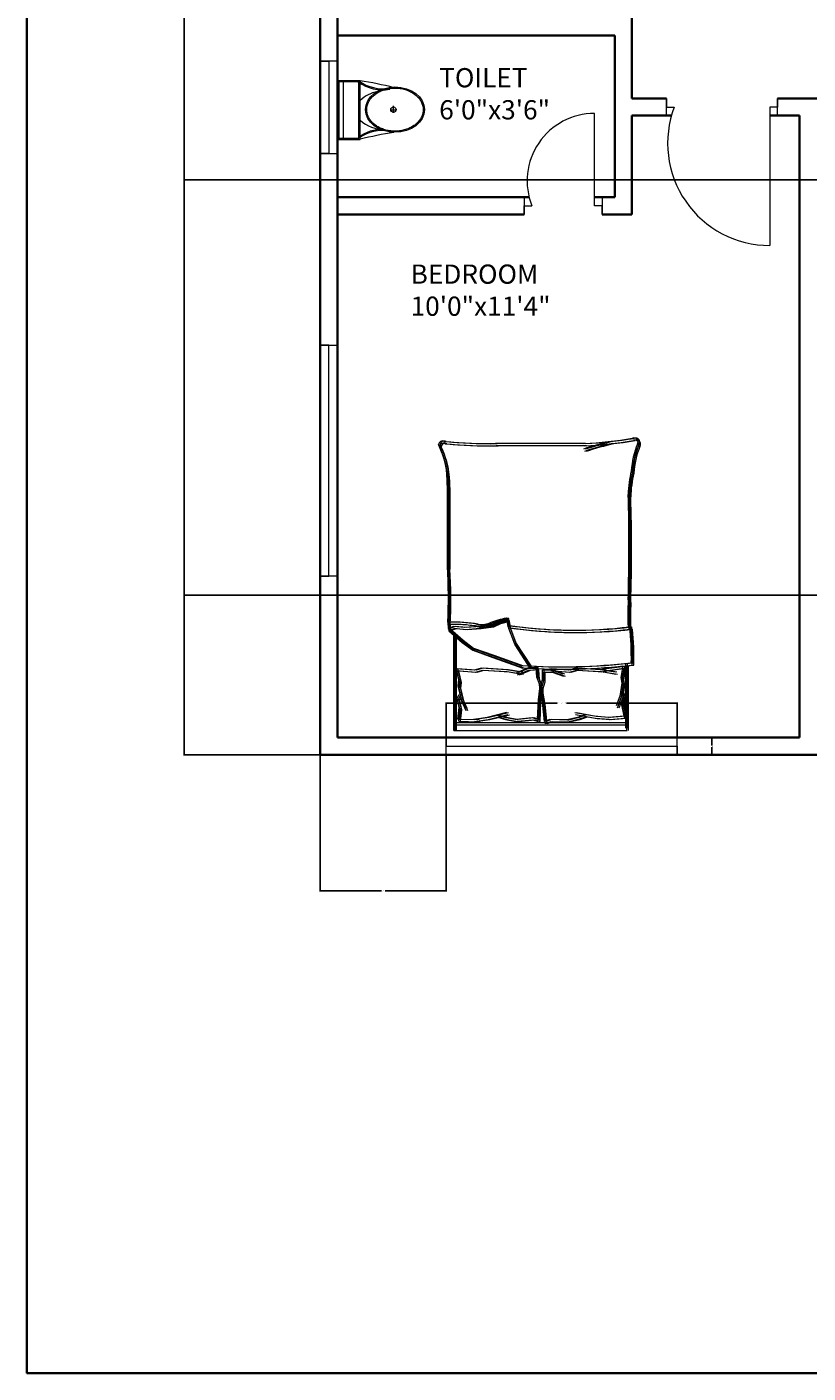
# Model space of a CAD drawing. Units: inches. Extents: x 2234 to 3001, y 1541 to 2386.
# Tile 1 of 12: x 2234 to 2437, y 1541 to 1891. Entities that reach past the tile are written whole.
import ezdxf

# ---------------------------------------------------------------- set-up
doc = ezdxf.new("R2010")
doc.units = ezdxf.units.IN
for name, color, linetype, lineweight in [('A-ANNO-DIMS', 2, 'Continuous', 18), ('A-ANNO-TTLB', 7, 'Continuous', 35), ('A-AREA-IDEN', 7, 'Continuous', 18), ('A-DOOR', 3, 'Continuous', 18), ('A-FLOR-FIXT', 9, 'Continuous', 18), ('A-FURN', 9, 'Continuous', 13), ('A-GLAZ', 4, 'Continuous', 18), ('A-WALL', 7, 'Continuous', 35)]:
    doc.layers.add(name, color=color, linetype=linetype, lineweight=lineweight)
doc.styles.get("Standard").update_dxf_attribs({"font": 'arial.ttf'})
doc.dimstyles.get("Standard").update_dxf_attribs({"dimtxt": 0.18, "dimasz": 0.18, "dimexe": 0.18, "dimexo": 0.0625, "dimgap": 0.09, "dimtad": 0, "dimtih": 1, "dimtoh": 1, "dimdec": 4, "dimzin": 0, "dimdsep": 46, "dimtxsty": 'Standard', "dimcen": 0.09, "dimadec": 0, "dimazin": 0, "dimtfac": 1, "dimtdec": 4, "dimtofl": 0, "dimtmove": 0, "dimatfit": 3, "dimfxl": 1, "dimtolj": 1, "dimtzin": 0, "dimarcsym": 0})

# ---------------------------------------------------------------- blocks, each defined once
blk = doc.blocks.new('A$C31115884')
for p, q in [((283, 498), (223, 498)), ((258, 466), (258, 523)), ((0, 200), (0, 0)), ((520, 200), (0, 200)), ((10, 190), (10, 10)), ((510, 190), (10, 190)), ((510, 10), (510, 190)), ((520, 0), (520, 200)), ((510, 54), (0, 54)), ((10, 10), (510, 10)), ((0, 0), (520, 0))]:
    blk.add_line(p, q)
blk.add_circle((256, 496), 23.6)
for centre, radius, start, end in [((2778, -205), 2807, 165.4549, 171.7133), ((3237, 905), 2807, 188.2867, 194.5451), ((-295, 403), 365, 324.2091, 9.3499), ((-295, 403), 375, 324.2091, 9.3499), ((139, 406), 293, 315.8436, 2.6563), ((806, 403), 375, 179.2036, 215.7909), ((806, 403), 365, 170.6501, 215.7909), ((384, 406), 293, 190.2774, 224.1564)]:
    blk.add_arc(centre, radius, start, end)
blk.add_ellipse((256, 510), major_axis=(0, -261), ratio=0.772727)
blk.add_open_spline([(256, 259), (263, 259), (270, 260), (288, 262), (299, 265), (320, 273), (330, 278), (350, 291), (360, 299), (378, 316), (386, 326), (402, 347), (409, 358), (421, 383), (427, 395), (436, 422), (440, 436), (445, 465), (447, 480), (448, 509), (448, 524), (445, 553), (443, 568), (436, 596), (432, 610), (422, 636), (416, 649), (402, 672), (395, 683), (379, 703), (370, 712), (351, 728), (341, 735), (321, 746), (310, 751), (289, 757), (278, 759), (256, 761), (245, 761), (223, 757), (212, 754), (191, 746), (181, 741), (161, 728), (151, 720), (133, 703), (125, 693), (110, 672), (103, 660), (90, 636), (85, 623), (76, 596), (72, 582), (67, 553), (66, 538), (64, 509), (65, 494), (68, 465), (70, 450), (77, 422), (81, 408), (91, 382), (97, 370), (111, 346), (118, 335), (135, 316), (144, 307), (162, 291), (172, 284), (193, 273), (203, 269), (225, 262), (236, 260), (250, 259), (253, 259), (256, 259)], degree=3, knots=[0, 0, 0, 0, 0.110105, 0.110105, 0.285049, 0.285049, 0.459994, 0.459994, 0.634938, 0.634938, 0.809882, 0.809882, 0.984827, 0.984827, 1.159771, 1.159771, 1.334715, 1.334715, 1.50966, 1.50966, 1.684604, 1.684604, 1.859549, 1.859549, 2.034493, 2.034493, 2.209437, 2.209437, 2.384382, 2.384382, 2.559326, 2.559326, 2.73427, 2.73427, 2.909215, 2.909215, 3.084159, 3.084159, 3.259103, 3.259103, 3.434048, 3.434048, 3.608992, 3.608992, 3.783936, 3.783936, 3.958881, 3.958881, 4.133825, 4.133825, 4.30877, 4.30877, 4.483714, 4.483714, 4.658658, 4.658658, 4.833603, 4.833603, 5.008547, 5.008547, 5.183491, 5.183491, 5.358436, 5.358436, 5.53338, 5.53338, 5.708324, 5.708324, 5.883269, 5.883269, 6.058213, 6.058213, 6.233158, 6.233158, 6.283185, 6.283185, 6.283185, 6.283185])
blk = doc.blocks.new('WIN-60-A')
for p, q in [((0, 60), (4.5, 60)), ((4.5, 60), (2.25, 60)), ((2.25, 60), (2.25, 0)), ((2.25, 0), (0, 0)), ((0, 0), (4.5, 0))]:
    blk.add_line(p, q)
blk = doc.blocks.new('WIN-60-B')
for p, q in [((0, 60), (4.5, 60)), ((4.5, 60), (2.25, 60)), ((2.25, 60), (2.25, 0)), ((4.5, 0), (0, 0)), ((2.25, 0), (4.5, 0))]:
    blk.add_line(p, q)
blk = doc.blocks.new('WIN-24-B')
for p, q in [((4.5, 24), (0, 24)), ((0, 24), (2.25, 24)), ((2.25, 24), (2.25, 0)), ((2.25, 0), (0, 0)), ((0, 0), (4.5, 0))]:
    blk.add_line(p, q)
blk = doc.blocks.new('BED-DOUBLE-B')
for p, q in [((37.77, 74.61), (14.78, 74.61)), ((37.77, 74.61), (14.78, 74.61)), ((37.98, 74.02), (15, 74.02)), ((37.98, 74.02), (15, 74.02)), ((38.22, 74.59), (15.24, 74.59)), ((38.22, 74.59), (15.24, 74.59)), ((38.44, 73.99), (15.45, 73.99)), ((38.44, 73.99), (15.46, 73.99)), ((2.39, 28.15), (2.47, 26.53, 3.61)), ((2.39, 28.15), (2.47, 26.53, 3.61)), ((2.85, 28.13), (2.92, 26.5, 3.61)), ((2.85, 28.13), (2.93, 26.5, 3.61)), ((15.47, 28.4), (13.59, 27.54)), ((15.47, 28.4), (13.59, 27.54)), ((15.93, 28.38), (14.05, 27.52)), ((15.93, 28.38), (14.05, 27.52)), ((17.79, 28.98), (15.47, 28.4)), ((17.79, 28.98), (15.47, 28.4)), ((18, 28.38), (15.68, 27.81)), ((18, 28.38), (15.69, 27.81)), ((18.24, 28.96), (15.93, 28.38)), ((18.24, 28.96), (15.93, 28.38)), ((18.46, 28.36), (16.14, 27.79)), ((18.46, 28.36), (16.14, 27.79)), ((18.07, 27.1), (17.79, 28.98)), ((18.07, 27.1), (17.79, 28.98)), ((18.29, 26.51), (18, 28.38)), ((18.29, 26.51), (18, 28.38)), ((18.53, 27.08), (18.24, 28.96)), ((18.53, 27.08), (18.24, 28.96)), ((18.75, 26.49), (18.46, 28.36)), ((18.75, 26.49), (18.46, 28.36)), ((3.9, 27.1), (2.47, 26.53)), ((3.9, 27.1), (2.47, 26.53)), ((2.47, 26.53), (5.93, 23.49)), ((2.47, 26.53), (5.93, 23.49)), ((2.61, 27.56), (2.68, 25.93, 3.61)), ((2.61, 27.56), (2.68, 25.93, 3.61)), ((4.12, 26.51), (2.68, 25.93)), ((4.12, 26.51), (2.68, 25.93)), ((2.68, 25.93), (6.14, 22.89)), ((2.68, 25.93), (6.14, 22.89)), ((4.36, 27.08), (2.92, 26.5)), ((2.92, 26.5), (6.38, 23.47)), ((4.36, 27.08), (2.93, 26.5)), ((2.93, 26.5), (6.39, 23.47)), ((3.06, 27.54), (3.14, 25.91, 3.61)), ((3.06, 27.54), (3.14, 25.91, 3.61)), ((4.57, 26.49), (3.14, 25.91)), ((4.57, 26.49), (3.14, 25.91)), ((3.14, 25.91), (6.6, 22.87)), ((3.14, 25.91), (6.6, 22.87)), ((6.79, 26.81), (3.9, 27.1)), ((6.8, 26.81), (3.9, 27.1)), ((3.96, 0.62), (3.96, 25.46)), ((3.96, 0.62), (3.96, 25.46)), ((7.01, 26.22), (4.12, 26.51)), ((7.01, 26.22), (4.12, 26.51)), ((4.18, 0.02), (4.18, 24.87)), ((4.18, 0.02), (4.18, 24.87)), ((7.25, 26.79), (4.36, 27.08)), ((7.25, 26.79), (4.36, 27.08)), ((4.42, 0.6), (4.42, 25.44)), ((4.42, 0.6), (4.42, 25.44)), ((7.47, 26.2), (4.57, 26.49)), ((7.47, 26.2), (4.57, 26.49)), ((4.63, 0), (4.63, 24.85)), ((4.63, 0), (4.63, 24.85)), ((10.41, 27.1), (6.79, 26.81)), ((10.41, 27.1), (6.8, 26.81)), ((10.62, 26.51), (7.01, 26.22)), ((10.62, 26.51), (7.01, 26.22)), ((10.87, 27.08), (7.25, 26.79)), ((10.87, 27.08), (7.25, 26.79)), ((11.08, 26.49), (7.47, 26.2)), ((11.08, 26.49), (7.47, 26.2)), ((13.59, 27.54), (10.41, 27.1)), ((13.59, 27.54), (10.41, 27.1)), ((13.8, 26.94), (10.62, 26.51)), ((13.81, 26.94), (10.62, 26.51)), ((14.05, 27.52), (10.87, 27.08)), ((14.05, 27.52), (10.87, 27.08)), ((14.26, 26.92), (11.08, 26.49)), ((14.26, 26.92), (11.08, 26.49)), ((15.68, 27.81), (13.8, 26.94)), ((15.69, 27.81), (13.81, 26.94)), ((16.14, 27.79), (14.26, 26.92)), ((16.14, 27.79), (14.26, 26.92)), ((19.67, 22.91), (18.07, 27.1)), ((19.67, 22.91), (18.07, 27.1)), ((19.88, 22.32), (18.29, 26.51)), ((19.88, 22.32), (18.29, 26.51)), ((20.12, 22.89), (18.53, 27.08)), ((20.12, 22.89), (18.53, 27.08)), ((20.34, 22.29), (18.75, 26.49)), ((20.34, 22.29), (18.75, 26.49)), ((5.93, 23.49), (8.67, 21.47)), ((5.93, 23.49), (8.68, 21.47)), ((6.14, 22.89), (8.89, 20.87)), ((6.14, 22.89), (8.89, 20.87)), ((6.38, 23.47), (9.13, 21.45)), ((6.39, 23.47), (9.13, 21.45)), ((6.6, 22.87), (9.35, 20.85)), ((6.6, 22.87), (9.35, 20.85)), ((8.67, 21.47), (13.88, 19.59)), ((8.68, 21.47), (13.88, 19.59)), ((9.13, 21.45), (14.34, 19.57)), ((9.13, 21.45), (14.34, 19.57)), ((23.58, 16.85), (19.67, 22.91)), ((23.58, 16.85), (19.67, 22.91)), ((23.79, 16.25), (19.88, 22.32)), ((23.79, 16.25), (19.88, 22.32)), ((24.04, 16.83), (20.12, 22.89)), ((24.04, 16.83), (20.12, 22.89)), ((24.25, 16.23), (20.34, 22.29)), ((24.25, 16.23), (20.34, 22.29)), ((8.89, 20.87), (14.09, 18.99)), ((8.89, 20.87), (14.09, 18.99)), ((9.35, 20.85), (14.55, 18.97)), ((9.35, 20.85), (14.55, 18.97)), ((13.88, 19.59), (21.67, 16.85)), ((13.88, 19.59), (21.67, 16.85)), ((14.09, 18.99), (21.88, 16.25)), ((14.09, 18.99), (21.88, 16.25)), ((14.34, 19.57), (22.12, 16.83)), ((14.34, 19.57), (22.12, 16.83)), ((14.55, 18.97), (22.34, 16.23)), ((14.55, 18.97), (22.34, 16.23)), ((48.59, 17.53), (48.59, 0.62)), ((48.59, 17.53), (48.59, 0.62)), ((49.05, 17.51), (49.05, 0.6)), ((49.05, 17.51), (49.05, 0.6)), ((9.28, 15.72), (4.49, 16.09)), ((4.49, 16.09), (5.22, 13.16)), ((9.29, 15.72), (4.49, 16.09)), ((4.49, 16.09), (5.22, 13.16)), ((9.5, 15.12), (4.71, 15.5)), ((4.71, 15.5), (5.43, 12.56)), ((9.5, 15.12), (4.71, 15.5)), ((4.71, 15.5), (5.43, 12.56)), ((9.74, 15.69), (4.95, 16.07)), ((4.95, 16.07), (5.67, 13.14)), ((9.74, 15.69), (4.95, 16.07)), ((4.95, 16.07), (5.67, 13.14)), ((9.96, 15.1), (5.16, 15.47)), ((5.16, 15.47), (5.89, 12.54)), ((9.96, 15.1), (5.16, 15.47)), ((5.16, 15.47), (5.89, 12.54)), ((11.12, 16.24), (9.28, 15.72)), ((11.12, 16.24), (9.29, 15.72)), ((11.33, 15.64), (9.5, 15.12)), ((11.33, 15.64), (9.5, 15.12)), ((11.57, 16.21), (9.74, 15.69)), ((11.57, 16.21), (9.74, 15.69)), ((11.79, 15.62), (9.96, 15.1)), ((11.79, 15.62), (9.96, 15.1)), ((17.66, 15.83), (11.12, 16.24)), ((17.66, 15.83), (11.12, 16.24)), ((17.87, 15.24), (11.33, 15.64)), ((17.87, 15.24), (11.33, 15.64)), ((18.12, 15.81), (11.57, 16.21)), ((18.12, 15.81), (11.57, 16.21)), ((18.33, 15.22), (11.79, 15.62)), ((18.33, 15.22), (11.79, 15.62)), ((21.43, 15.21), (17.66, 15.83)), ((21.43, 15.21), (17.66, 15.83)), ((21.64, 14.61), (17.87, 15.24)), ((21.64, 14.61), (17.87, 15.24)), ((21.88, 15.19), (18.12, 15.81)), ((21.88, 15.19), (18.12, 15.81)), ((22.1, 14.59), (18.33, 15.22)), ((22.1, 14.59), (18.33, 15.22)), ((23.12, 16.25), (20.25, 15.05)), ((23.12, 16.25), (20.25, 15.05)), ((23.33, 15.65), (20.47, 14.45)), ((23.33, 15.65), (20.47, 14.45)), ((23.58, 16.23), (20.71, 15.03)), ((23.58, 16.23), (20.71, 15.03)), ((23.79, 15.63), (20.92, 14.43)), ((23.79, 15.63), (20.92, 14.43)), ((25.41, 16.39), (23.12, 16.25)), ((25.41, 16.39), (23.12, 16.25)), ((25.62, 15.79), (23.33, 15.65)), ((25.62, 15.79), (23.33, 15.65)), ((25.87, 16.37), (23.58, 16.23)), ((25.87, 16.37), (23.58, 16.23)), ((26.08, 15.77), (23.79, 15.63)), ((26.08, 15.77), (23.79, 15.63)), ((25.57, 13.89), (25.41, 16.39)), ((25.57, 13.89), (25.41, 16.39)), ((25.78, 13.3), (25.62, 15.79)), ((25.78, 13.3), (25.62, 15.79)), ((26.02, 13.87), (25.87, 16.37)), ((26.02, 13.87), (25.87, 16.37)), ((26.24, 13.27), (26.08, 15.77)), ((26.24, 13.27), (26.08, 15.77)), ((27.03, 13.3), (27.03, 15.8)), ((27.03, 15.8), (29.33, 15.8)), ((27.03, 13.3), (27.03, 15.8)), ((27.03, 15.8), (29.33, 15.8)), ((27.24, 12.7), (27.24, 15.21)), ((27.24, 15.21), (29.54, 15.21)), ((27.24, 12.7), (27.24, 15.21)), ((27.24, 15.21), (29.54, 15.21)), ((27.49, 13.28), (27.49, 15.78)), ((27.49, 15.78), (29.78, 15.78)), ((27.49, 13.28), (27.49, 15.78)), ((27.49, 15.78), (29.78, 15.78)), ((27.7, 12.68), (27.7, 15.19)), ((27.7, 15.19), (30, 15.19)), ((27.7, 12.68), (27.7, 15.19)), ((27.7, 15.19), (30, 15.19)), ((33.73, 15.72), (28.94, 16.09)), ((33.73, 15.72), (28.94, 16.09)), ((33.95, 15.12), (29.15, 15.5)), ((33.95, 15.12), (29.15, 15.5)), ((29.33, 15.8), (32.26, 14.78)), ((29.33, 15.8), (32.26, 14.78)), ((34.19, 15.69), (29.4, 16.07)), ((34.19, 15.69), (29.4, 16.07)), ((29.54, 15.21), (32.48, 14.19)), ((29.54, 15.21), (32.48, 14.19)), ((34.4, 15.1), (29.61, 15.47)), ((34.4, 15.1), (29.61, 15.47)), ((29.78, 15.78), (32.72, 14.76)), ((29.78, 15.78), (32.72, 14.76)), ((30, 15.19), (32.93, 14.17)), ((30, 15.19), (32.93, 14.17)), ((35.56, 16.24), (33.73, 15.72)), ((35.56, 16.24), (33.73, 15.72)), ((35.78, 15.64), (33.95, 15.12)), ((35.78, 15.64), (33.95, 15.12)), ((36.02, 16.21), (34.19, 15.69)), ((36.02, 16.21), (34.19, 15.69)), ((36.23, 15.62), (34.4, 15.1)), ((36.23, 15.62), (34.4, 15.1)), ((42.11, 15.83), (35.56, 16.24)), ((42.11, 15.83), (35.56, 16.24)), ((42.32, 15.24), (35.78, 15.64)), ((42.32, 15.24), (35.78, 15.64)), ((42.57, 15.81), (36.02, 16.21)), ((42.57, 15.81), (36.02, 16.21)), ((42.78, 15.22), (36.23, 15.62)), ((42.78, 15.22), (36.23, 15.62)), ((42.11, 15.83), (43.17, 16.13)), ((42.11, 15.83), (43.17, 16.13)), ((45.87, 15.21), (42.11, 15.83)), ((45.87, 15.21), (42.11, 15.83)), ((42.32, 15.24), (43.38, 15.54)), ((42.32, 15.24), (43.38, 15.54)), ((46.09, 14.61), (42.32, 15.24)), ((46.09, 14.61), (42.32, 15.24)), ((42.57, 15.81), (43.62, 16.11)), ((42.57, 15.81), (43.62, 16.11)), ((46.33, 15.19), (42.57, 15.81)), ((46.33, 15.19), (42.57, 15.81)), ((42.78, 15.22), (43.84, 15.52)), ((42.78, 15.22), (43.84, 15.52)), ((46.54, 14.59), (42.78, 15.22)), ((46.54, 14.59), (42.78, 15.22)), ((43.17, 16.13), (47.93, 16.81)), ((43.17, 16.13), (47.93, 16.81)), ((43.38, 15.54), (48.14, 16.21)), ((43.38, 15.54), (48.14, 16.21)), ((43.62, 16.11), (48.38, 16.79)), ((43.62, 16.11), (48.38, 16.79)), ((43.84, 15.52), (48.6, 16.19)), ((43.84, 15.52), (48.6, 16.19)), ((47.93, 16.81), (47.39, 13.84)), ((47.93, 16.81), (47.39, 13.84)), ((48.14, 16.21), (47.6, 13.24)), ((48.14, 16.21), (47.6, 13.24)), ((48.38, 16.79), (47.84, 13.82)), ((48.38, 16.79), (47.84, 13.82)), ((48.6, 16.19), (48.06, 13.22)), ((48.6, 16.19), (48.06, 13.22)), ((48.8, 16.93), (48.8, 0.02)), ((48.8, 16.93), (48.8, 0.02)), ((49.26, 16.91), (49.26, 0)), ((49.26, 16.91), (49.26, 0)), ((5.22, 13.16), (5.04, 11.66)), ((5.22, 13.16), (5.04, 11.66)), ((5.04, 11.66), (5.79, 8.33)), ((5.04, 11.66), (5.79, 8.33)), ((5.43, 12.56), (5.25, 11.07)), ((5.43, 12.56), (5.25, 11.07)), ((5.25, 11.07), (6, 7.73)), ((5.25, 11.07), (6, 7.73)), ((5.67, 13.14), (5.5, 11.64)), ((5.67, 13.14), (5.5, 11.64)), ((5.5, 11.64), (6.25, 8.31)), ((5.5, 11.64), (6.25, 8.31)), ((5.89, 12.54), (5.71, 11.04)), ((5.89, 12.54), (5.71, 11.04)), ((5.71, 11.04), (6.46, 7.71)), ((5.71, 11.04), (6.46, 7.71)), ((26.21, 12.17), (25.57, 13.89)), ((26.21, 12.17), (25.57, 13.89)), ((26.43, 11.58), (25.78, 13.3)), ((26.43, 11.58), (25.78, 13.3)), ((25.94, 7.96), (26.29, 10.96)), ((25.94, 7.96), (26.29, 10.96)), ((26.67, 12.15), (26.02, 13.87)), ((26.67, 12.15), (26.02, 13.87)), ((26.29, 10.96), (26.21, 12.17)), ((26.29, 10.96), (26.21, 12.17)), ((26.88, 11.56), (26.24, 13.27)), ((26.89, 11.56), (26.24, 13.27)), ((26.39, 7.94), (26.75, 10.94)), ((26.39, 7.94), (26.75, 10.94)), ((26.5, 10.36), (26.43, 11.58)), ((26.5, 10.36), (26.43, 11.58)), ((26.49, 11.54), (27.03, 13.3)), ((26.49, 11.54), (27.03, 13.3)), ((26.49, 10.33), (26.49, 11.54)), ((26.49, 10.33), (26.49, 11.54)), ((26.75, 10.94), (26.67, 12.15)), ((26.75, 10.94), (26.67, 12.15)), ((26.7, 10.95), (27.24, 12.7)), ((26.7, 10.95), (27.24, 12.7)), ((26.7, 9.73), (26.7, 10.95)), ((26.7, 9.73), (26.7, 10.95)), ((26.96, 10.34), (26.88, 11.56)), ((26.96, 10.34), (26.89, 11.56)), ((26.95, 11.52), (27.49, 13.28)), ((26.95, 11.52), (27.49, 13.28)), ((26.95, 10.31), (26.95, 11.52)), ((26.95, 10.31), (26.95, 11.52)), ((27.16, 10.93), (27.7, 12.68)), ((27.16, 10.93), (27.7, 12.68)), ((27.16, 9.71), (27.16, 10.93)), ((27.16, 9.71), (27.16, 10.93)), ((47.66, 12.35), (47.12, 8.98)), ((47.66, 12.35), (47.12, 8.98)), ((47.87, 11.76), (47.33, 8.38)), ((47.87, 11.76), (47.33, 8.38)), ((47.39, 13.84), (47.66, 12.35)), ((47.39, 13.84), (47.66, 12.35)), ((48.11, 12.33), (47.57, 8.96)), ((48.11, 12.33), (47.57, 8.96)), ((47.6, 13.24), (47.87, 11.76)), ((47.6, 13.24), (47.87, 11.76)), ((48.33, 11.74), (47.79, 8.36)), ((48.33, 11.74), (47.79, 8.36)), ((47.84, 13.82), (48.11, 12.33)), ((47.84, 13.82), (48.11, 12.33)), ((48.06, 13.22), (48.33, 11.74)), ((48.06, 13.22), (48.33, 11.74)), ((4.84, 8.4), (5.32, 9.38)), ((4.84, 8.4), (5.32, 9.38)), ((5.39, 6), (4.84, 8.4)), ((5.39, 6), (4.84, 8.4)), ((5.05, 7.81), (5.53, 8.78)), ((5.05, 7.81), (5.53, 8.78)), ((5.61, 5.41), (5.05, 7.81)), ((5.61, 5.41), (5.05, 7.81)), ((5.3, 8.38), (5.78, 9.36)), ((5.3, 8.38), (5.78, 9.36)), ((5.85, 5.98), (5.3, 8.38)), ((5.85, 5.98), (5.3, 8.38)), ((5.51, 7.79), (5.99, 8.76)), ((5.51, 7.79), (5.99, 8.76)), ((6.06, 5.39), (5.51, 7.79)), ((6.07, 5.39), (5.51, 7.79)), ((5.79, 8.33), (6.89, 5.83)), ((5.79, 8.33), (6.89, 5.83)), ((6, 7.73), (7.11, 5.23)), ((6, 7.73), (7.11, 5.23)), ((6.25, 8.31), (7.35, 5.81)), ((6.25, 8.31), (7.35, 5.81)), ((6.46, 7.71), (7.56, 5.21)), ((6.46, 7.71), (7.56, 5.21)), ((25.71, 2.94), (25.94, 7.96)), ((25.71, 2.94), (25.94, 7.96)), ((25.92, 2.35), (26.15, 7.37)), ((25.92, 2.35), (26.15, 7.37)), ((26.15, 7.37), (26.5, 10.36)), ((26.15, 7.37), (26.5, 10.36)), ((26.17, 2.92), (26.39, 7.94)), ((26.17, 2.92), (26.39, 7.94)), ((26.38, 2.33), (26.61, 7.35)), ((26.38, 2.33), (26.61, 7.35)), ((27.03, 7.36), (26.49, 10.33)), ((27.03, 7.36), (26.49, 10.33)), ((26.61, 7.35), (26.96, 10.34)), ((26.61, 7.35), (26.96, 10.34)), ((27.24, 6.76), (26.7, 9.73)), ((27.24, 6.76), (26.7, 9.73)), ((27.49, 7.34), (26.95, 10.31)), ((27.49, 7.34), (26.95, 10.31)), ((27.57, 2.36), (27.03, 7.36)), ((27.57, 2.36), (27.03, 7.36)), ((27.7, 6.74), (27.16, 9.71)), ((27.7, 6.74), (27.16, 9.71)), ((28.03, 2.34), (27.49, 7.34)), ((28.03, 2.34), (27.49, 7.34)), ((47.12, 8.98), (46.17, 6.41)), ((47.12, 8.98), (46.17, 6.41)), ((47.33, 8.38), (46.38, 5.82)), ((47.33, 8.38), (46.38, 5.82)), ((47.57, 8.96), (46.63, 6.39)), ((47.57, 8.96), (46.63, 6.39)), ((47.79, 8.36), (46.84, 5.8)), ((47.79, 8.36), (46.84, 5.8)), ((48.06, 9.11), (47.52, 10.06)), ((48.06, 9.11), (47.52, 10.06)), ((47.66, 6.68), (48.06, 9.11)), ((47.66, 6.68), (48.06, 9.11)), ((48.27, 8.52), (47.73, 9.46)), ((48.27, 8.52), (47.73, 9.46)), ((47.87, 6.09), (48.27, 8.52)), ((47.87, 6.09), (48.27, 8.52)), ((48.52, 9.09), (47.98, 10.04)), ((48.52, 9.09), (47.98, 10.04)), ((48.11, 6.66), (48.52, 9.09)), ((48.11, 6.66), (48.52, 9.09)), ((48.73, 8.5), (48.19, 9.44)), ((48.73, 8.5), (48.19, 9.44)), ((48.33, 6.07), (48.73, 8.5)), ((48.33, 6.07), (48.73, 8.5)), ((5.04, 3.01), (5.39, 6)), ((5.04, 3.01), (5.39, 6)), ((5.25, 2.41), (5.61, 5.41)), ((5.25, 2.41), (5.61, 5.41)), ((5.5, 2.98), (5.85, 5.98)), ((5.5, 2.98), (5.85, 5.98)), ((5.71, 2.39), (6.06, 5.39)), ((5.71, 2.39), (6.07, 5.39)), ((12.69, 3.48), (17.76, 4.75)), ((12.7, 3.48), (17.76, 4.75)), ((12.91, 2.89), (17.97, 4.15)), ((12.91, 2.89), (17.97, 4.15)), ((13.15, 3.46), (18.21, 4.73)), ((13.15, 3.46), (18.21, 4.73)), ((13.37, 2.87), (18.43, 4.13)), ((13.37, 2.87), (18.43, 4.13)), ((15.23, 4.05), (17.16, 3.49)), ((15.23, 4.05), (17.16, 3.49)), ((15.69, 4.03), (17.61, 3.47)), ((15.69, 4.03), (17.62, 3.47)), ((27.78, 1.77), (27.24, 6.76)), ((27.78, 1.77), (27.24, 6.76)), ((28.24, 1.75), (27.7, 6.74)), ((28.24, 1.75), (27.7, 6.74)), ((40.53, 3.71), (35.4, 4.66)), ((40.53, 3.71), (35.4, 4.66)), ((40.74, 3.12), (35.61, 4.06)), ((40.74, 3.12), (35.61, 4.06)), ((40.98, 3.69), (35.85, 4.64)), ((40.98, 3.69), (35.85, 4.64)), ((37.96, 4.12), (36.07, 3.44)), ((37.96, 4.12), (36.07, 3.44)), ((41.2, 3.1), (36.07, 4.04)), ((41.2, 3.1), (36.07, 4.04)), ((38.17, 3.52), (36.29, 2.85)), ((38.18, 3.52), (36.29, 2.85)), ((38.42, 4.1), (36.53, 3.42)), ((38.42, 4.1), (36.53, 3.42)), ((38.63, 3.5), (36.74, 2.83)), ((38.63, 3.5), (36.74, 2.83)), ((44.1, 3.44), (40.53, 3.71)), ((44.1, 3.44), (40.53, 3.71)), ((44.55, 3.42), (40.98, 3.69)), ((44.55, 3.42), (40.98, 3.69)), ((48.19, 3.73), (44.19, 3.43)), ((48.19, 3.73), (44.2, 3.43)), ((48.65, 3.71), (44.65, 3.41)), ((48.65, 3.71), (44.65, 3.41)), ((48.2, 3.71), (47.66, 6.68)), ((48.2, 3.71), (47.66, 6.68)), ((48.41, 3.12), (47.87, 6.09)), ((48.41, 3.12), (47.87, 6.09)), ((48.65, 3.69), (48.11, 6.66)), ((48.65, 3.69), (48.11, 6.66)), ((48.87, 3.1), (48.33, 6.07)), ((48.87, 3.1), (48.33, 6.07)), ((48.59, 2.05), (3.96, 2.05)), ((48.59, 2.05), (3.96, 2.05)), ((3.96, 0.02), (3.96, 0.62)), ((3.96, 0.02), (48.59, 0.02)), ((48.8, 1.45), (4.18, 1.45)), ((48.8, 1.45), (4.18, 1.45)), ((49.05, 2.03), (4.42, 2.03)), ((49.05, 2.03), (4.42, 2.03)), ((4.42, 0), (4.42, 0.6)), ((49.26, 1.43), (4.63, 1.43)), ((49.26, 1.43), (4.63, 1.43)), ((5.04, 3.01), (10.08, 2.91)), ((5.04, 3.01), (10.09, 2.91)), ((5.25, 2.41), (10.3, 2.32)), ((5.25, 2.41), (10.3, 2.32)), ((5.5, 2.98), (10.54, 2.89)), ((5.5, 2.98), (10.54, 2.89)), ((5.71, 2.39), (10.76, 2.3)), ((5.71, 2.39), (10.76, 2.3)), ((9.15, 2.99), (12.69, 3.48)), ((9.15, 2.99), (12.7, 3.48)), ((10.08, 2.91), (9.15, 2.99)), ((10.09, 2.91), (9.15, 2.99)), ((9.36, 2.39), (12.91, 2.89)), ((9.36, 2.39), (12.91, 2.89)), ((10.3, 2.32), (9.36, 2.39)), ((10.3, 2.32), (9.36, 2.39)), ((9.61, 2.97), (13.15, 3.46)), ((9.61, 2.97), (13.15, 3.46)), ((10.54, 2.89), (9.61, 2.97)), ((10.54, 2.89), (9.61, 2.97)), ((9.82, 2.37), (13.37, 2.87)), ((9.82, 2.37), (13.37, 2.87)), ((10.76, 2.3), (9.82, 2.37)), ((10.76, 2.3), (9.82, 2.37)), ((15.44, 3.45), (17.37, 2.89)), ((15.44, 3.45), (17.37, 2.89)), ((15.9, 3.43), (17.83, 2.87)), ((15.9, 3.43), (17.83, 2.87)), ((17.16, 3.49), (19.89, 2.99)), ((17.16, 3.49), (19.89, 2.99)), ((17.37, 2.89), (20.11, 2.39)), ((17.37, 2.89), (20.11, 2.39)), ((17.61, 3.47), (20.35, 2.97)), ((17.62, 3.47), (20.35, 2.97)), ((17.83, 2.87), (20.56, 2.37)), ((17.83, 2.87), (20.56, 2.37)), ((19.89, 2.99), (20.19, 3.01)), ((19.89, 2.99), (20.19, 3.01)), ((20.11, 2.39), (20.41, 2.41)), ((20.11, 2.39), (20.41, 2.41)), ((20.19, 3.01), (24.33, 3.4)), ((20.19, 3.01), (24.33, 3.4)), ((20.35, 2.97), (20.65, 2.98)), ((20.35, 2.97), (20.65, 2.98)), ((20.41, 2.41), (24.54, 2.8)), ((20.41, 2.41), (24.54, 2.8)), ((20.56, 2.37), (20.86, 2.39)), ((20.56, 2.37), (20.86, 2.39)), ((20.65, 2.98), (24.79, 3.38)), ((20.65, 2.98), (24.79, 3.38)), ((20.86, 2.39), (25, 2.78)), ((20.86, 2.39), (25, 2.78)), ((24.33, 3.4), (25.71, 2.94)), ((24.33, 3.4), (25.71, 2.94)), ((24.54, 2.8), (25.92, 2.35)), ((24.54, 2.8), (25.92, 2.35)), ((24.79, 3.38), (26.17, 2.92)), ((24.79, 3.38), (26.17, 2.92)), ((25, 2.78), (26.38, 2.33)), ((25, 2.78), (26.38, 2.33)), ((28.92, 2.9), (27.57, 2.36)), ((28.92, 2.9), (27.57, 2.36)), ((29.13, 2.31), (27.78, 1.77)), ((29.13, 2.31), (27.78, 1.77)), ((29.38, 2.88), (28.03, 2.34)), ((29.38, 2.88), (28.03, 2.34)), ((29.59, 2.29), (28.24, 1.75)), ((29.59, 2.29), (28.24, 1.75)), ((33.07, 2.77), (28.92, 2.9)), ((33.07, 2.77), (28.92, 2.9)), ((33.29, 2.17), (29.13, 2.31)), ((33.29, 2.17), (29.13, 2.31)), ((33.53, 2.75), (29.38, 2.88)), ((33.53, 2.75), (29.38, 2.88)), ((33.74, 2.15), (29.59, 2.29)), ((33.74, 2.15), (29.59, 2.29)), ((33.37, 2.77), (33.07, 2.77)), ((33.37, 2.77), (33.07, 2.77)), ((33.59, 2.17), (33.29, 2.17)), ((33.59, 2.17), (33.29, 2.17)), ((36.07, 3.44), (33.37, 2.77)), ((36.07, 3.44), (33.37, 2.77)), ((33.83, 2.75), (33.53, 2.75)), ((33.83, 2.75), (33.53, 2.75)), ((36.29, 2.85), (33.59, 2.17)), ((36.29, 2.85), (33.59, 2.17)), ((34.04, 2.15), (33.74, 2.15)), ((34.04, 2.15), (33.74, 2.15)), ((36.53, 3.42), (33.83, 2.75)), ((36.53, 3.42), (33.83, 2.75)), ((36.74, 2.83), (34.04, 2.15)), ((36.74, 2.83), (34.04, 2.15)), ((44.31, 2.85), (40.74, 3.12)), ((44.31, 2.85), (40.74, 3.12)), ((44.77, 2.83), (41.2, 3.1)), ((44.77, 2.83), (41.2, 3.1)), ((44.19, 3.43), (44.1, 3.44)), ((44.2, 3.43), (44.1, 3.44)), ((44.41, 2.83), (44.31, 2.85)), ((44.41, 2.83), (44.31, 2.85)), ((48.41, 3.14), (44.41, 2.83)), ((48.41, 3.14), (44.41, 2.83)), ((44.65, 3.41), (44.55, 3.42)), ((44.65, 3.41), (44.55, 3.42)), ((44.87, 2.81), (44.77, 2.83)), ((44.87, 2.81), (44.77, 2.83)), ((48.86, 3.12), (44.87, 2.81)), ((48.86, 3.12), (44.87, 2.81)), ((4.42, 0), (49.05, 0))]:
    blk.add_line(p, q)
for centre, radius, start, end in [((1.03, 74.26), 1.03, 62.6588, 176.02), ((1.03, 74.26), 1.03, 62.6588, 176.02), ((-19.28, 64.73), 21.54, 357.4714, 26.4681), ((-19.28, 64.73), 21.54, 357.4714, 26.4681), ((1.24, 73.67), 1.03, 62.6588, 176.02), ((1.24, 73.67), 1.03, 62.6588, 176.02), ((-19.07, 64.14), 21.54, 357.4714, 26.4681), ((-19.07, 64.14), 21.54, 357.4714, 26.4681), ((1.48, 74.24), 1.03, 62.6588, 176.02), ((1.49, 74.24), 1.03, 62.6588, 176.02), ((-18.82, 64.71), 21.54, 357.4714, 26.4681), ((-18.82, 64.71), 21.54, 357.4714, 26.4681), ((1.7, 73.64), 1.03, 62.6588, 176.02), ((1.7, 73.64), 1.03, 62.6588, 176.02), ((-18.61, 64.12), 21.54, 357.4714, 26.4681), ((-18.61, 64.12), 21.54, 357.4714, 26.4681), ((13.41, 198.83), 124.23, 264.4998, 270.6351), ((13.41, 198.83), 124.23, 264.4998, 270.6351), ((13.62, 198.23), 124.23, 264.4998, 270.6351), ((13.62, 198.23), 124.23, 264.4998, 270.6351), ((13.86, 198.81), 124.23, 264.4998, 270.6351), ((13.86, 198.81), 124.23, 264.4998, 270.6351), ((14.08, 198.21), 124.23, 264.4998, 270.6351), ((14.08, 198.21), 124.23, 264.4998, 270.6351), ((67.91, -21.52), 99.41, 103.3832, 107.7053), ((67.91, -21.52), 99.41, 103.3832, 107.7053), ((31.83, 188.15), 113.69, 272.9958, 279.4091), ((31.83, 188.15), 113.69, 272.9958, 279.4091), ((68.13, -22.12), 99.41, 103.3832, 107.7053), ((68.13, -22.12), 99.41, 103.3832, 107.7053), ((32.04, 187.55), 113.69, 272.9958, 279.4091), ((32.04, 187.55), 113.69, 272.9958, 279.4091), ((68.37, -21.54), 99.41, 103.3832, 107.7053), ((68.37, -21.54), 99.41, 103.3832, 107.7053), ((32.28, 188.13), 113.69, 272.9958, 279.4091), ((32.28, 188.13), 113.69, 272.9958, 279.4091), ((68.58, -22.14), 99.41, 103.3832, 107.7053), ((68.58, -22.14), 99.41, 103.3832, 107.7053), ((32.5, 187.53), 113.69, 272.9958, 279.4091), ((32.5, 187.53), 113.69, 272.9958, 279.4091), ((72.06, 66.24), 22, 157.9751, 176.652), ((72.06, 66.24), 22, 157.9751, 176.652), ((72.27, 65.64), 22, 157.9751, 176.652), ((72.27, 65.64), 22, 157.9751, 176.652), ((50.82, 75.05), 1.02, 326.1736, 113.4781), ((50.82, 75.05), 1.02, 326.1736, 113.4781), ((72.51, 66.22), 22, 157.9751, 176.652), ((72.51, 66.22), 22, 157.9751, 176.652), ((51.03, 74.46), 1.02, 326.1736, 113.4781), ((51.03, 74.46), 1.02, 326.1736, 113.4781), ((72.73, 65.62), 22, 157.9751, 176.652), ((72.73, 65.62), 22, 157.9751, 176.652), ((51.27, 75.03), 1.02, 326.1736, 113.4781), ((51.27, 75.03), 1.02, 326.1736, 113.4781), ((51.49, 74.44), 1.02, 326.1736, 113.4781), ((51.49, 74.44), 1.02, 326.1736, 113.4781), ((76.95, 60.86), 27.67, 166.0648, 178.9113), ((76.95, 60.86), 27.67, 166.0648, 178.9113), ((77.16, 60.26), 27.67, 166.0648, 178.9113), ((77.16, 60.26), 27.67, 166.0648, 178.9113), ((77.41, 60.84), 27.67, 166.0648, 178.9113), ((77.41, 60.84), 27.67, 166.0648, 178.9113), ((77.62, 60.24), 27.67, 166.0648, 178.9113), ((77.62, 60.24), 27.67, 166.0648, 178.9113), ((4261.85, 63.95), 4259.62, 180.00217, 180.28689), ((4261.85, 63.95), 4259.62, 180.00217, 180.28689), ((4262.07, 63.35), 4259.62, 180.00217, 180.28689), ((4262.07, 63.35), 4259.62, 180.00217, 180.28689), ((4262.31, 63.92), 4259.62, 180.00217, 180.28689), ((4262.31, 63.92), 4259.62, 180.00217, 180.28689), ((4262.53, 63.33), 4259.62, 180.00217, 180.28689), ((4262.53, 63.33), 4259.62, 180.00217, 180.28689), ((-400.87, 47.88), 450.36, 358.2277, 1.7185), ((-400.87, 47.88), 450.36, 358.2277, 1.7185), ((-400.66, 47.28), 450.36, 358.2277, 1.7185), ((-400.66, 47.28), 450.36, 358.2277, 1.7185), ((-400.41, 47.86), 450.36, 358.2277, 1.7185), ((-400.41, 47.86), 450.36, 358.2277, 1.7185), ((-400.2, 47.26), 450.36, 358.2277, 1.7185), ((-400.2, 47.26), 450.36, 358.2277, 1.7185), ((-118.36, 34.53), 120.92, 356.9791, 3.8365), ((-118.36, 34.53), 120.92, 356.9791, 3.8365), ((-118.14, 33.93), 120.92, 356.9791, 3.8365), ((-118.14, 33.93), 120.92, 356.9791, 3.8365), ((-117.9, 34.51), 120.92, 356.9791, 3.8365), ((-117.9, 34.51), 120.92, 356.9791, 3.8365), ((-117.69, 33.91), 120.92, 356.9791, 3.8365), ((-117.69, 33.91), 120.92, 356.9791, 3.8365), ((208.05, 29.73), 158.84, 178.4762, 181.0082), ((208.06, 29.73), 158.84, 178.4762, 181.0082), ((208.27, 29.13), 158.84, 178.4762, 181.0082), ((208.27, 29.13), 158.84, 178.4762, 181.0082), ((208.51, 29.7), 158.84, 178.4762, 181.0082), ((208.51, 29.7), 158.84, 178.4762, 181.0082), ((208.73, 29.11), 158.84, 178.4762, 181.0082), ((208.73, 29.11), 158.84, 178.4762, 181.0082), ((3.91, -5.6), 33.79, 79.8763, 92.5657), ((3.91, -5.6), 33.79, 79.8763, 92.5657), ((4.36, -5.62), 33.79, 79.8763, 92.5657), ((4.36, -5.62), 33.79, 79.8763, 92.5657), ((10.99, 33.36), 5.81, 258.6608, 293.7384), ((10.99, 33.36), 5.81, 258.6608, 293.7384), ((11.44, 33.34), 5.81, 258.6608, 293.7384), ((11.44, 33.34), 5.81, 258.6608, 293.7384), ((22.74, 2), 27.69, 100.6617, 109.8806), ((22.74, 2), 27.69, 100.6617, 109.8806), ((22.96, 1.4), 27.69, 100.6617, 109.8806), ((22.96, 1.4), 27.69, 100.6617, 109.8806), ((23.2, 1.98), 27.69, 100.6617, 109.8806), ((23.2, 1.98), 27.69, 100.6617, 109.8806), ((23.41, 1.38), 27.69, 100.6617, 109.8806), ((23.41, 1.38), 27.69, 100.6617, 109.8806), ((17.62, 29.04), 0.172, 340.2464, 91.1377), ((17.62, 29.04), 0.172, 340.2464, 91.1377), ((17.84, 28.44), 0.172, 340.2464, 91.1377), ((17.84, 28.44), 0.172, 340.2464, 91.1377), ((18.08, 29.02), 0.172, 340.2464, 91.1377), ((18.08, 29.02), 0.172, 340.2464, 91.1377), ((18.29, 28.42), 0.172, 340.2464, 91.1377), ((18.29, 28.42), 0.172, 340.2464, 91.1377), ((4.12, -6.19), 33.79, 79.8763, 92.5657), ((4.12, -6.19), 33.79, 79.8763, 92.5657), ((4.58, -6.22), 33.79, 79.8763, 92.5657), ((4.58, -6.22), 33.79, 79.8763, 92.5657), ((11.2, 32.76), 5.81, 258.6608, 293.7384), ((11.2, 32.76), 5.81, 258.6608, 293.7384), ((11.66, 32.74), 5.81, 258.6608, 293.7384), ((11.66, 32.74), 5.81, 258.6608, 293.7384), ((35.25, 146.58), 120.47, 261.7845, 276.9006), ((35.25, 146.58), 120.47, 261.7845, 276.9006), ((35.47, 145.98), 120.47, 261.7845, 276.9006), ((35.47, 145.98), 120.47, 261.7845, 276.9006), ((35.71, 146.56), 120.47, 261.7845, 276.9006), ((35.71, 146.56), 120.47, 261.7845, 276.9006), ((35.92, 145.96), 120.47, 261.7845, 276.9006), ((35.92, 145.96), 120.47, 261.7845, 276.9006), ((-27.69, 19.38), 77.79, 358.7218, 5.604), ((-27.69, 19.38), 77.79, 358.7218, 5.604), ((-27.47, 18.79), 77.79, 358.7218, 5.604), ((-27.47, 18.79), 77.79, 358.7218, 5.604), ((-27.23, 19.36), 77.79, 358.7218, 5.604), ((-27.23, 19.36), 77.79, 358.7218, 5.604), ((-27.02, 18.76), 77.79, 358.7218, 5.604), ((-27.02, 18.76), 77.79, 358.7218, 5.604), ((31.89, 170.61), 154.04, 266.0865, 276.7821), ((31.89, 170.61), 154.04, 266.0865, 276.7821), ((32.35, 170.59), 154.04, 266.0865, 276.7821), ((32.35, 170.59), 154.04, 266.0865, 276.7821), ((32.1, 170.01), 154.04, 266.0865, 276.7821), ((32.1, 170.01), 154.04, 266.0865, 276.7821), ((32.56, 169.99), 154.04, 266.0865, 276.7821), ((32.56, 169.99), 154.04, 266.0865, 276.7821)]:
    blk.add_arc(centre, radius, start, end)
blk = doc.blocks.new('*D25')
at = {"layer": 'A-ANNO-DIMS', "color": 0, "lineweight": -2, "transparency": 16777216}
for p, q in [((2342.51, 1706.67), (2342.51, 1715.79)), ((2342.69, 1715.61), (2371.27, 1715.61)), ((2402.33, 1715.61), (2373.75, 1715.61)), ((2402.51, 1706.67), (2402.51, 1715.79))]:
    blk.add_line(p, q, dxfattribs=at)
at = {"layer": 'A-ANNO-DIMS', "color": 0, "transparency": 16777216}
for points in [[(2342.69, 1715.64), (2342.69, 1715.58), (2342.51, 1715.61)], [(2402.33, 1715.64), (2402.33, 1715.58), (2402.51, 1715.61)]]:
    blk.add_solid(points, dxfattribs=at)
at = {"layer": 'Defpoints', "color": 0, "transparency": 16777216}
for p in [(2342.51, 1715.61), (2342.51, 1706.61), (2402.51, 1706.61)]:
    blk.add_point(p, dxfattribs=at)
at = {"layer": 'A-ANNO-DIMS', "color": 0, "transparency": 16777216, "insert": (2372.51, 1715.61), "char_height": 0.18, "attachment_point": 5}
blk.add_mtext('\\A1;WINDOW A 60 TYP.', dxfattribs=at)
blk = doc.blocks.new('*D26')
at = {"layer": 'A-ANNO-DIMS', "color": 0, "lineweight": -2, "transparency": 16777216}
for p, q in [((2402.57, 1706.61), (2411.69, 1706.61)), ((2411.51, 1706.43), (2411.51, 1704.54)), ((2411.51, 1702.29), (2411.51, 1704.18)), ((2402.57, 1702.11), (2411.69, 1702.11))]:
    blk.add_line(p, q, dxfattribs=at)
at = {"layer": 'A-ANNO-DIMS', "color": 0, "transparency": 16777216}
for points in [[(2411.48, 1706.43), (2411.54, 1706.43), (2411.51, 1706.61)], [(2411.48, 1702.29), (2411.54, 1702.29), (2411.51, 1702.11)]]:
    blk.add_solid(points, dxfattribs=at)
at = {"layer": 'Defpoints', "color": 0, "transparency": 16777216}
for p in [(2402.51, 1706.61), (2411.51, 1706.61), (2402.51, 1702.11)]:
    blk.add_point(p, dxfattribs=at)
at = {"layer": 'A-ANNO-DIMS', "color": 0, "transparency": 16777216, "insert": (2411.51, 1704.36), "char_height": 0.18, "attachment_point": 5}
blk.add_mtext('\\A1;5 TYP.', dxfattribs=at)
blk = doc.blocks.new('*D63')
at = {"layer": 'A-ANNO-DIMS', "color": 0, "lineweight": -2, "transparency": 16777216}
for p, q in [((2314.19, 2000.11), (2274.22, 2000.11)), ((2274.4, 1999.93), (2274.4, 1851.29)), ((2274.4, 1702.29), (2274.4, 1850.93)), ((2309.69, 1702.11), (2274.22, 1702.11))]:
    blk.add_line(p, q, dxfattribs=at)
at = {"layer": 'A-ANNO-DIMS', "color": 0, "transparency": 16777216}
for points in [[(2274.37, 1999.93), (2274.43, 1999.93), (2274.4, 2000.11)], [(2274.37, 1702.29), (2274.43, 1702.29), (2274.4, 1702.11)]]:
    blk.add_solid(points, dxfattribs=at)
at = {"layer": 'Defpoints', "color": 0, "transparency": 16777216}
for p in [(2274.4, 2000.11), (2314.25, 2000.11), (2309.75, 1702.11)]:
    blk.add_point(p, dxfattribs=at)
at = {"layer": 'A-ANNO-DIMS', "color": 0, "transparency": 16777216, "insert": (2274.4, 1851.11), "char_height": 0.18, "attachment_point": 5}
blk.add_mtext('\\A1;298', dxfattribs=at)
blk = doc.blocks.new('*D65')
at = {"layer": 'A-ANNO-DIMS', "color": 0, "lineweight": -2, "transparency": 16777216}
for p, q in [((2634.69, 1851.65), (2274.22, 1851.65)), ((2274.4, 1851.47), (2274.4, 1797.83)), ((2274.4, 1743.83), (2274.4, 1797.47)), ((2634.69, 1743.65), (2274.22, 1743.65))]:
    blk.add_line(p, q, dxfattribs=at)
at = {"layer": 'A-ANNO-DIMS', "color": 0, "transparency": 16777216}
for points in [[(2274.37, 1851.47), (2274.43, 1851.47), (2274.4, 1851.65)], [(2274.37, 1743.83), (2274.43, 1743.83), (2274.4, 1743.65)]]:
    blk.add_solid(points, dxfattribs=at)
at = {"layer": 'Defpoints', "color": 0, "transparency": 16777216}
for p in [(2274.4, 1851.65), (2634.75, 1851.65), (2634.75, 1743.65)]:
    blk.add_point(p, dxfattribs=at)
at = {"layer": 'A-ANNO-DIMS', "color": 0, "transparency": 16777216, "insert": (2274.4, 1797.65), "char_height": 0.18, "attachment_point": 5}
blk.add_mtext('\\A1;108', dxfattribs=at)
blk = doc.blocks.new('*D69')
at = {"layer": 'A-ANNO-DIMS', "color": 0, "lineweight": -2, "transparency": 16777216}
for p, q in [((2309.75, 1702.05), (2309.75, 1666.58)), ((2342.51, 1702.05), (2342.51, 1666.58)), ((2309.93, 1666.76), (2325.67, 1666.76)), ((2342.33, 1666.76), (2326.59, 1666.76))]:
    blk.add_line(p, q, dxfattribs=at)
at = {"layer": 'A-ANNO-DIMS', "color": 0, "transparency": 16777216}
for points in [[(2309.93, 1666.79), (2309.93, 1666.73), (2309.75, 1666.76)], [(2342.33, 1666.79), (2342.33, 1666.73), (2342.51, 1666.76)]]:
    blk.add_solid(points, dxfattribs=at)
at = {"layer": 'Defpoints', "color": 0, "transparency": 16777216}
for p in [(2309.75, 1702.11), (2342.51, 1702.11), (2342.51, 1666.76)]:
    blk.add_point(p, dxfattribs=at)
at = {"layer": 'A-ANNO-DIMS', "color": 0, "transparency": 16777216, "insert": (2326.13, 1666.76), "char_height": 0.18, "attachment_point": 5}
blk.add_mtext('\\A1;32.756', dxfattribs=at)

msp = doc.modelspace()

# ---------------------------------------------------------------- linework, layer by layer
at = {"layer": 'A-ANNO-TTLB'}
msp.add_lwpolyline([(2233.5367, 2385.7012), (3001.3383, 2385.7012), (3001.3383, 1541.435), (2233.5367, 1541.435)], close=True, dxfattribs=at)
at = {"layer": 'A-DOOR'}
for p, q in [((2399.7528, 1868.2928), (2399.7528, 1872.7928)), ((2399.7528, 1872.7928), (2399.7528, 1870.5428)), ((2428.5694, 1868.2928), (2428.5694, 1872.7928)), ((2428.5694, 1872.7928), (2428.5694, 1870.5428)), ((2381.0207, 1844.861), (2381.0207, 1868.861)), ((2399.7528, 1870.5428), (2401.7528, 1870.5428)), ((2428.5694, 1870.5428), (2426.5694, 1870.5428)), ((2426.5694, 1870.5428), (2426.5694, 1834.5428)), ((2362.732, 1847.111), (2362.732, 1842.611)), ((2362.732, 1842.611), (2362.732, 1844.861)), ((2362.732, 1844.861), (2364.732, 1844.861)), ((2383.0207, 1844.861), (2381.0207, 1844.861)), ((2383.0207, 1847.111), (2383.0207, 1842.611)), ((2383.0207, 1842.611), (2383.0207, 1844.861))]:
    msp.add_line(p, q, dxfattribs=at)
for centre, radius, start, end in [((2381.0207, 1851.3334), 17.5276, 90, 201.670679), ((2426.5694, 1861.0964), 26.5537, 159.160869, 270)]:
    msp.add_arc(centre, radius, start, end, dxfattribs=at)
at = {"layer": 'A-WALL'}
for p, q in [((2309.7534, 2298.611), (2309.7534, 1702.111)), ((2314.2534, 2069.111), (2314.2534, 1706.611)), ((2390.7534, 1897.2352), (2390.7534, 1872.7928)), ((2314.2534, 1889.111), (2386.2534, 1889.111)), ((2386.2534, 1847.111), (2386.2534, 1889.111)), ((2399.7528, 1872.7928), (2390.7534, 1872.7928)), ((2443.517, 1872.7928), (2428.5694, 1872.7928)), ((2390.7534, 1868.2928), (2401.0095, 1868.2928)), ((2390.7534, 1868.2928), (2390.7534, 1842.611)), ((2426.5694, 1868.2928), (2434.2534, 1868.2928)), ((2434.2534, 1868.2928), (2434.2534, 1842.611)), ((2314.2534, 1847.111), (2364.0094, 1847.111)), ((2381.0207, 1847.111), (2386.2534, 1847.111)), ((2314.2534, 1842.611), (2362.732, 1842.611)), ((2314.2534, 1842.611), (2362.732, 1842.611)), ((2314.2534, 1842.611), (2362.732, 1842.611)), ((2383.0207, 1842.611), (2390.7534, 1842.611)), ((2383.0207, 1842.611), (2390.7534, 1842.611)), ((2383.0207, 1842.611), (2386.2534, 1842.611)), ((2434.2534, 1842.611), (2434.2534, 1706.611)), ((2434.2534, 1706.611), (2314.2534, 1706.611)), ((2888.2534, 1702.111), (2309.7534, 1702.111))]:
    msp.add_line(p, q, dxfattribs=at)

# ---------------------------------------------------------------- block references
at = {"layer": 'A-FLOR-FIXT', "xscale": 0.0292470664339069, "yscale": 0.0292470664339069, "zscale": 0.0292470664339069, "rotation": 270}
msp.add_blockref('A$C31115884', (2314.2534, 1877.3489), dxfattribs=at)
at = {"layer": 'A-FURN'}
msp.add_blockref('BED-DOUBLE-B', (2340.484, 1708.445), dxfattribs=at)
at = {"layer": 'A-GLAZ'}
msp.add_blockref('WIN-24-B', (2309.753, 1858.4577), dxfattribs=at)
for name, p, rotation in [('WIN-60-B', (2314.2539, 1808.6196), 180), ('WIN-60-A', (2402.5088, 1702.1106), 90)]:
    msp.add_blockref(name, p, dxfattribs=dict(at, rotation=rotation))

# ---------------------------------------------------------------- texts
at = {"layer": 'A-AREA-IDEN', "char_height": 5, "attachment_point": 1}
for s, width, insert in [('TOILET\\P6\'0"x3\'6"', 62.366049, (2340.6602, 1880.655)), ('BEDROOM\\P10\'0"x11\'4"', 118.657606, (2333.2275, 1829.6011))]:
    msp.add_mtext_dynamic_manual_height_columns(s, width=width, gutter_width=12.5, heights=[0], dxfattribs=dict(at, insert=insert))

# ---------------------------------------------------------------- dimensions: what is measured, and where the dimension line sits
at = {"layer": 'A-ANNO-DIMS'}
for base, p1, p2, picture, middle in [((2274.4034, 2000.111), (2309.7534, 1702.111), (2314.2534, 2000.111), '*D63', (2274.4034, 1851.111)), ((2274.4034, 1851.6488), (2634.7534, 1743.6488), (2634.7534, 1851.6488), '*D65', (2274.4034, 1797.6488))]:
    dim = msp.add_linear_dim(base=base, p1=p1, p2=p2, angle=90, dimstyle='Standard', override={"dimdec": 0, "dimlfac": 1, "dimrnd": 0, "dimzin": 0, "dimdsep": 46, "dimlunit": 2}, dxfattribs=at)
    dim.commit()
    dim.dimension.update_dxf_attribs({"geometry": picture, "text_midpoint": middle})
for base, p1, p2, angle, text, picture, middle in [((2342.5091, 1715.611), (2402.5091, 1706.611), (2342.5091, 1706.611), 180, 'WINDOW A <> TYP.', '*D25', (2372.5091, 1715.611)), ((2411.5091161305, 1706.6110170859), (2402.5091161305, 1702.1110170859), (2402.5091161305, 1706.6110170859), 90, '<> TYP.', '*D26', (2411.5091161305, 1704.3610170859))]:
    dim = msp.add_linear_dim(base=base, p1=p1, p2=p2, angle=angle, text=text, dimstyle='Standard', override={"dimdec": 0, "dimlfac": 1, "dimrnd": 0, "dimzin": 0, "dimdsep": 46, "dimlunit": 2}, dxfattribs=at)
    dim.commit()
    dim.dimension.update_dxf_attribs({"geometry": picture, "text_midpoint": middle})
dim = msp.add_linear_dim(base=(2342.5091, 1666.761), p1=(2309.7534, 1702.111), p2=(2342.5091, 1702.111), dimstyle='Standard', override={"dimdec": 3, "dimlfac": 1, "dimrnd": 0, "dimzin": 0, "dimdsep": 46, "dimlunit": 2}, dxfattribs=at)
dim.commit()
dim.dimension.update_dxf_attribs({"geometry": '*D69', "text_midpoint": (2326.1313, 1666.761)})

doc.saveas('drawing.dxf')
